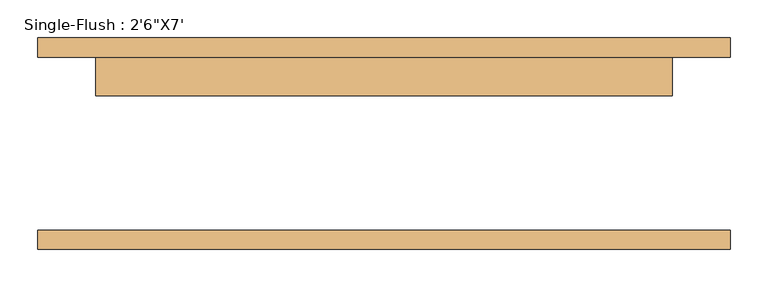
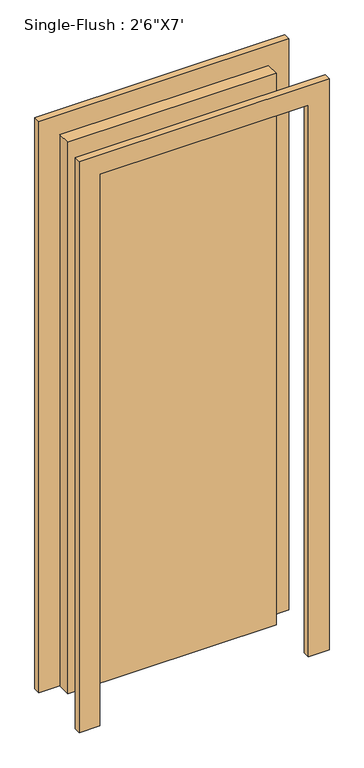
"""IFC4 building model written with IfcOpenShell, lengths in millimetres: door geometry."""

from ifc_helpers import new_model, si_unit, frame, origin, origin_with_axes, place, context, project, spatial, polyline, outline, extrude, source, transform, mapped, element, save


def door_bb98abfd(model_context):
    return source(origin(), model_context, "Body", "SweptSolid", [
        extrude(outline(polyline([(2209.8, -457.2), (0.0, -457.2), (0.0, -381.0), (2133.6, -381.0), (2133.6, 381.0), (0.0, 381.0), (0.0, 457.2), (2209.8, 457.2), (2209.8, -457.2)])), frame((0.0, 114.3, 0.0), z_axis=(0.0, 1.0, 0.0), x_axis=(0.0, 0.0, 1.0)), (0.0, 0.0, 1.0), 25.4),
        extrude(outline(polyline([(2209.8, 457.2), (2209.8, -457.2), (0.0, -457.2), (0.0, -381.0), (2133.6, -381.0), (2133.6, 381.0), (0.0, 381.0), (0.0, 457.2), (2209.8, 457.2)])), frame((0.0, -139.7, 0.0), z_axis=(0.0, 1.0, 0.0), x_axis=(0.0, 0.0, 1.0)), (0.0, 0.0, 1.0), 25.4),
        extrude(outline(polyline([(381.0, 63.5), (-381.0, 63.5), (-381.0, 114.3), (381.0, 114.3), (381.0, 63.5)])), origin_with_axes(), (0.0, 0.0, 1.0), 2133.6),
    ])


if __name__ == "__main__":
    model = new_model("IFC4")
    model_context = context("Model", 3, world=origin())
    ifc_project = project(units=[si_unit("LENGTHUNIT", "METRE", prefix="MILLI")], contexts=[model_context])
    site = spatial("IfcSite", under=ifc_project)
    building = spatial("IfcBuilding", under=site)
    placement = place(None, origin())
    door_shape = door_bb98abfd(model_context)
    element("IfcDoor", 1, ObjectType="Single-Flush : 2'6\"X7'", at=placement, inside=building, context=model_context, shape_type="MappedRepresentation", body=[
        mapped(door_shape, transform((0.0, 0.0, 0.0), x_axis=(1.0, 0.0, 0.0), y_axis=(0.0, 1.0, 0.0), z_axis=(0.0, 0.0, 1.0))),
    ])
    save(model, "model.ifc")

# Revit data of these elements
# Type "Single-Flush : 2'6\"X7'"
#   Type Mark = "9"
#   Construction Type Id = "MDOOR"
#   Assembly Code = "C1020"
#   Analytic Construction = "Metal"
#   Thickness = 0' - 2"
#   Heat Transfer Coefficient (U) = 0.651978 BTU/(h·ft²·°F)
#   Height = 7' - 0"
#   Trim Projection Ext = 0' - 1"
#   Trim Projection Int = 0' - 1"
#   Trim Width = 0' - 3"
#   Width = 2' - 6"
#   Define Thermal Properties by = 1
#   Door Material = Door - Panel
#   Frame Material = Door - Frame
#   Visual Light Transmittance = 0
#   Solar Heat Gain Coefficient = 0
#   Function = (empty or 0)
#   Wall Closure = (empty or 0)
# Element 1 (IfcDoor, "Single-Flush : 2'6\"X7'")
#   Materials on its faces: "Door - Frame", "Door - Panel"
# Materials
#   "Door - Panel": class "Wood", colour RGB 210 159 95, transparency 0, Cost = 0
#   "Door - Frame": colour RGB 118 70 51, transparency 0, Cost = 0
